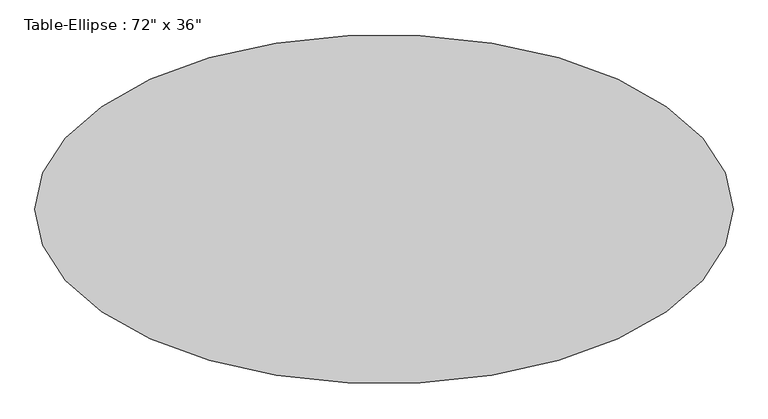
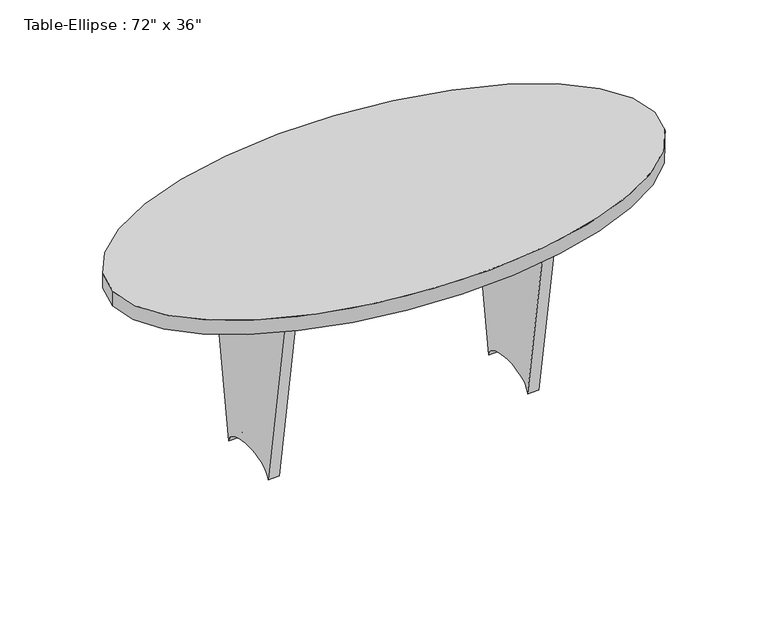
"""IFC4 building model written with IfcOpenShell, lengths in millimetres: furniture geometry."""

from ifc_helpers import new_model, si_unit, point, frame, origin, place, context, project, spatial, ellipse_curve, trimmed, source, transform, mapped, element, save
from ifc_brep_helpers import plane_surface, extruded_surface, advanced_brep


def furniture_027a2ad9(model_context):
    return source(origin(), model_context, "Body", "AdvancedBrep", [
        advanced_brep(
        [(-419.1, 19.05, 711.2), (419.1, 19.05, 711.2), (419.1, 19.05, 474.1333333), (-419.1, 19.05, 474.1333333), (-419.1, -19.05, 711.2), (-419.1, -19.05, 474.1333333), (419.1, -19.05, 474.1333333), (419.1, -19.05, 711.2)],
        [
            (0, 1),
            (1, 2),
            (2, 3, ellipse_curve(frame((0.0, 19.05, 474.1333333), z_axis=(0.0, -1.0, 0.0), x_axis=(1.0, 0.0, 0.0)), 419.1, 101.6)),
            (3, 0),
            (4, 5),
            (5, 6, ellipse_curve(frame((0.0, -19.05, 474.1333333), z_axis=(0.0, 1.0, 0.0), x_axis=(1.0, 0.0, 0.0)), 419.1, 101.6)),
            (6, 7),
            (7, 4),
            (0, 4),
            (7, 1),
            (6, 2),
            (5, 3),
        ],
        [
            plane_surface(frame((-419.1, 19.05, 711.2), z_axis=(0.0, 1.0, 0.0), x_axis=(1.0, 0.0, 0.0))),
            plane_surface(frame((-419.1, -19.05, 711.2), z_axis=(0.0, -1.0, 0.0), x_axis=(-1.0, 0.0, 0.0))),
            plane_surface(frame((-419.1, 19.05, 711.2), z_axis=(0.0, 0.0, 1.0), x_axis=(0.0, -1.0, 0.0))),
            plane_surface(frame((419.1, 19.05, 711.2), z_axis=(1.0, 0.0, 0.0), x_axis=(0.0, -1.0, 0.0))),
            extruded_surface(trimmed(ellipse_curve(frame((0.0, -57.15, 474.1333333), z_axis=(0.0, -1.0, 0.0), x_axis=(1.0, 0.0, 0.0)), 419.1, 101.6), [point((419.1, -57.15, 474.1333333))], [point((-419.1, -57.15, 474.1333333))], True, "CARTESIAN"), (0.0, 38.099999999999994, 0.0), 38.099999999999994),
            plane_surface(frame((-419.1, 19.05, 474.1333333), z_axis=(-1.0, 0.0, 0.0), x_axis=(0.0, -1.0, 0.0))),
        ],
        [
            (0, [[1, 2, 3, 4]]),
            (1, [[5, 6, 7, 8]]),
            (2, [[-1, 9, -8, 10]]),
            (3, [[-2, -10, -7, 11]]),
            (4, [[-3, -11, -6, 12]]),
            (5, [[-4, -12, -5, -9]]),
        ],
    ),
        advanced_brep(
        [(457.2, 228.6, 711.2), (457.2, -228.6, 711.2), (457.2, -114.3, 0.0), (457.2, 114.3, 0.0), (419.1, 228.6, 711.2), (419.1, 114.3, 0.0), (419.1, -114.3, 0.0), (419.1, -228.6, 711.2)],
        [
            (0, 1),
            (1, 2),
            (2, 3, ellipse_curve(frame((457.2, 0.0, 0.0), z_axis=(-1.0, 0.0, 0.0), x_axis=(0.0, 1.0, 0.0)), 114.3, 50.8)),
            (3, 0),
            (4, 5),
            (5, 6, ellipse_curve(frame((419.1, 0.0, 0.0), z_axis=(1.0, 0.0, 0.0), x_axis=(0.0, 1.0, 0.0)), 114.3, 50.8)),
            (6, 7),
            (7, 4),
            (0, 4),
            (7, 1),
            (6, 2),
            (5, 3),
        ],
        [
            plane_surface(frame((457.2, -228.6, 711.2), z_axis=(1.0, 0.0, 0.0), x_axis=(0.0, -1.0, 0.0))),
            plane_surface(frame((419.1, -228.6, 711.2), z_axis=(-1.0, 0.0, 0.0), x_axis=(0.0, 1.0, 0.0))),
            plane_surface(frame((457.2, 228.6, 711.2), z_axis=(0.0, 0.0, 1.0), x_axis=(-1.0, 0.0, 0.0))),
            plane_surface(frame((457.2, -228.6, 711.2), z_axis=(0.0, -0.9873303712766982, -0.158678095383759), x_axis=(-1.0, 0.0, 0.0))),
            extruded_surface(trimmed(ellipse_curve(frame((381.0, 0.0, 0.0), z_axis=(-1.0, 0.0, 0.0), x_axis=(0.0, 1.0, 0.0)), 114.3, 50.8), [point((381.0, -114.3, 0.0))], [point((381.0, 114.3, 0.0))], True, "CARTESIAN"), (38.10000000000002, 0.0, 0.0), 38.10000000000002),
            plane_surface(frame((457.2, 114.3, 0.0), z_axis=(0.0, 0.9873303712767002, -0.15867809538374666), x_axis=(-1.0, 0.0, 0.0))),
        ],
        [
            (0, [[1, 2, 3, 4]]),
            (1, [[5, 6, 7, 8]]),
            (2, [[-1, 9, -8, 10]]),
            (3, [[-2, -10, -7, 11]]),
            (4, [[-3, -11, -6, 12]]),
            (5, [[-4, -12, -5, -9]]),
        ],
    ),
        advanced_brep(
        [(-419.1, 228.6, 711.2), (-419.1, -228.6, 711.2), (-419.1, -114.3, 0.0), (-419.1, 114.3, 0.0), (-457.2, 228.6, 711.2), (-457.2, 114.3, 0.0), (-457.2, -114.3, 0.0), (-457.2, -228.6, 711.2)],
        [
            (0, 1),
            (1, 2),
            (2, 3, ellipse_curve(frame((-419.1, 0.0, 0.0), z_axis=(-1.0, 0.0, 0.0), x_axis=(0.0, 1.0, 0.0)), 114.3, 50.8)),
            (3, 0),
            (4, 5),
            (5, 6, ellipse_curve(frame((-457.2, 0.0, 0.0), z_axis=(1.0, 0.0, 0.0), x_axis=(0.0, 1.0, 0.0)), 114.3, 50.8)),
            (6, 7),
            (7, 4),
            (0, 4),
            (7, 1),
            (6, 2),
            (5, 3),
        ],
        [
            plane_surface(frame((-419.1, -228.6, 711.2), z_axis=(1.0, 0.0, 0.0), x_axis=(0.0, -1.0, 0.0))),
            plane_surface(frame((-457.2, -228.6, 711.2), z_axis=(-1.0, 0.0, 0.0), x_axis=(0.0, 1.0, 0.0))),
            plane_surface(frame((-419.1, 228.6, 711.2), z_axis=(0.0, 0.0, 1.0), x_axis=(-1.0, 0.0, 0.0))),
            plane_surface(frame((-419.1, -228.6, 711.2), z_axis=(0.0, -0.9873303712766983, -0.15867809538375854), x_axis=(-1.0, 0.0, 0.0))),
            extruded_surface(trimmed(ellipse_curve(frame((-495.3, 0.0, 0.0), z_axis=(-1.0, 0.0, 0.0), x_axis=(0.0, 1.0, 0.0)), 114.3, 50.8), [point((-495.3, -114.3, 0.0))], [point((-495.3, 114.3, 0.0))], True, "CARTESIAN"), (38.10000000000002, 0.0, 0.0), 38.10000000000002),
            plane_surface(frame((-419.1, 114.3, 0.0), z_axis=(0.0, 0.9873303712766998, -0.15867809538374977), x_axis=(-1.0, 0.0, 0.0))),
        ],
        [
            (0, [[1, 2, 3, 4]]),
            (1, [[5, 6, 7, 8]]),
            (2, [[-1, 9, -8, 10]]),
            (3, [[-2, -10, -7, 11]]),
            (4, [[-3, -11, -6, 12]]),
            (5, [[-4, -12, -5, -9]]),
        ],
    ),
        advanced_brep(
        [(-914.4, 0.0, 762.0), (914.4, 0.0, 762.0), (-914.4, 0.0, 711.2), (914.4, 0.0, 711.2)],
        [
            (0, 1, ellipse_curve(frame((0.0, 0.0, 762.0), z_axis=(0.0, 0.0, 1.0), x_axis=(1.0, 0.0, 0.0)), 914.4, 457.2)),
            (1, 0, ellipse_curve(frame((0.0, 0.0, 762.0), z_axis=(0.0, 0.0, 1.0), x_axis=(1.0, 0.0, 0.0)), 914.4, 457.2)),
            (2, 3, ellipse_curve(frame((0.0, 0.0, 711.2), z_axis=(0.0, 0.0, -1.0), x_axis=(1.0, 0.0, 0.0)), 914.4, 457.2)),
            (3, 2, ellipse_curve(frame((0.0, 0.0, 711.2), z_axis=(0.0, 0.0, -1.0), x_axis=(1.0, 0.0, 0.0)), 914.4, 457.2)),
            (0, 2),
            (3, 1),
        ],
        [
            plane_surface(frame((914.4, 0.0, 762.0), z_axis=(0.0, 0.0, 1.0), x_axis=(0.0, 1.0, 0.0))),
            plane_surface(frame((914.4, 0.0, 711.2), z_axis=(0.0, 0.0, -1.0), x_axis=(0.0, -1.0, 0.0))),
            extruded_surface(trimmed(ellipse_curve(frame((0.0, 0.0, 660.4), z_axis=(0.0, 0.0, 1.0), x_axis=(1.0, 0.0, 0.0)), 914.4, 457.2), [point((-914.4, 0.0, 660.4))], [point((914.4, 0.0, 660.4))], True, "CARTESIAN"), (0.0, 0.0, 50.80000000000007), 50.80000000000007),
            extruded_surface(trimmed(ellipse_curve(frame((0.0, 0.0, 660.4), z_axis=(0.0, 0.0, 1.0), x_axis=(1.0, 0.0, 0.0)), 914.4, 457.2), [point((914.4, 0.0, 660.4))], [point((-914.4, 0.0, 660.4))], True, "CARTESIAN"), (0.0, 0.0, 50.80000000000007), 50.80000000000007),
        ],
        [
            (0, [[1, 2]]),
            (1, [[3, 4]]),
            (2, [[-1, 5, -4, 6]]),
            (3, [[-2, -6, -3, -5]]),
        ],
    ),
    ])


if __name__ == "__main__":
    model = new_model("IFC4")
    model_context = context("Model", 3, world=origin())
    ifc_project = project(units=[si_unit("LENGTHUNIT", "METRE", prefix="MILLI")], contexts=[model_context])
    site = spatial("IfcSite", under=ifc_project)
    building = spatial("IfcBuilding", under=site)
    placement = place(None, origin())
    furniture_shape = furniture_027a2ad9(model_context)
    element("IfcFurniture", 1, ObjectType="Table-Ellipse : 72\" x 36\"", at=placement, inside=building, context=model_context, shape_type="MappedRepresentation", body=[
        mapped(furniture_shape, transform((0.0, 0.0, 0.0), x_axis=(1.0, 0.0, 0.0), y_axis=(0.0, 1.0, 0.0), z_axis=(0.0, 0.0, 1.0))),
    ])
    save(model, "model.ifc")

# Revit data of these elements
# Type "Table-Ellipse : 72\" x 36\""
#   Assembly Code = "E2020200"
#   Half Width = 1' - 6"
#   Half Length = 3' - 0"
#   Height = 2' - 6"
#   Length = 6' - 0"
#   Width = 3' - 0"
#   Base Material = Birch
#   Top Material = Gypsum Wall Board
#   Default Elevation = 0
# Element 1 (IfcFurniture, "Table-Ellipse : 72\" x 36\"")
#   Materials on its faces: "Birch", "Gypsum Wall Board"
# Materials
#   "Birch": class "Wood", colour RGB 224 178 126, transparency 0, Description = "Betula Alleghaniensis", Cost = 0
#   "Gypsum Wall Board": class "Generic", colour RGB 127 127 127, transparency 0, Description = "Gypsum Wall Board", Cost = 0
